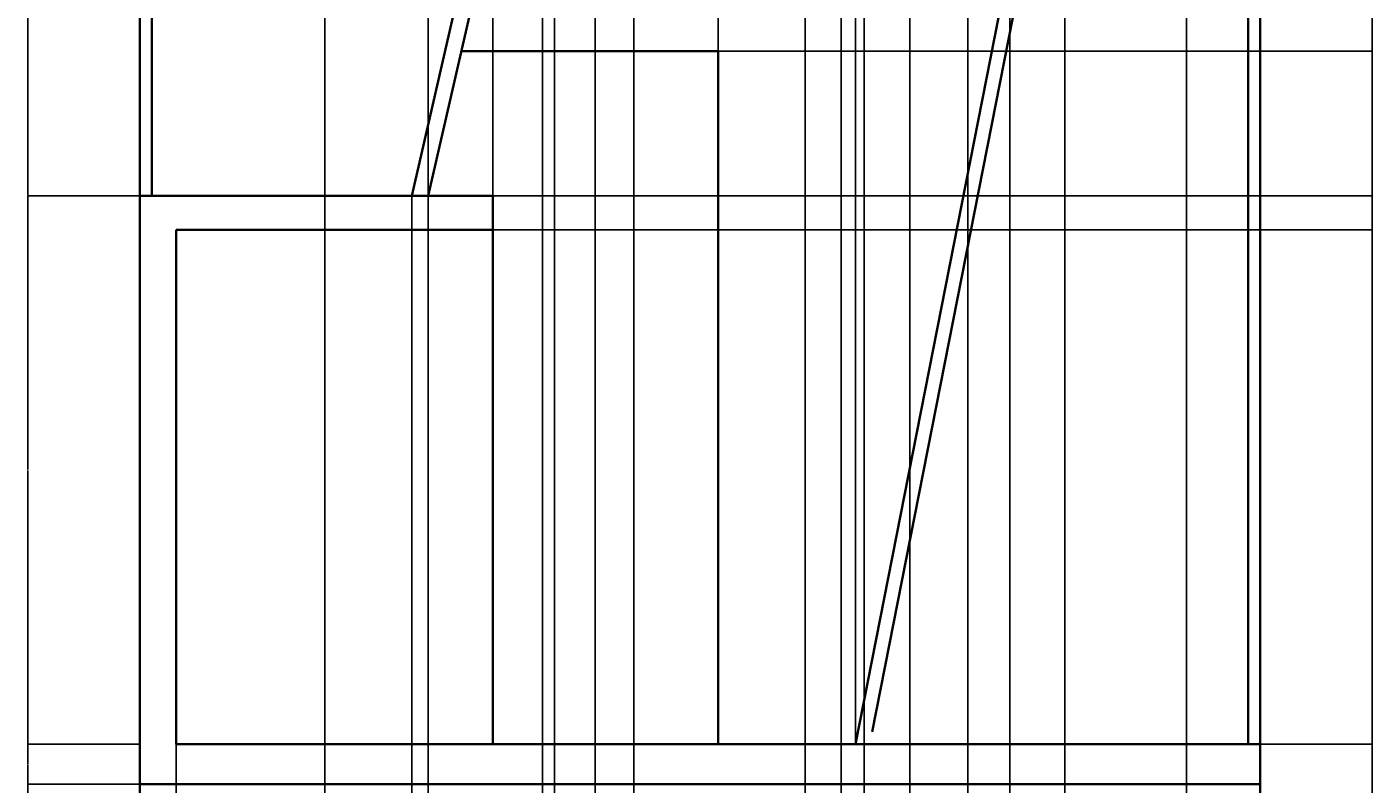
# Model space of a CAD drawing. Units: feet. Extents: x 2373 to 3800, y 799 to 1842.
# Tile 3 of 4: x 3224 to 3800, y 1129 to 1453. Entities that reach past the tile are written whole.
import ezdxf

# ---------------------------------------------------------------- set-up
doc = ezdxf.new("R2010")
doc.units = ezdxf.units.FT
doc.layers.add('A-ANNO-DIMS', color=2, linetype='Continuous', lineweight=18)
doc.layers.add('A-ELEV', color=7, linetype='Continuous', lineweight=35)
doc.styles.get("Standard").update_dxf_attribs({"font": 'arial.ttf'})
doc.dimstyles.get("Standard").update_dxf_attribs({"dimtxt": 0.18, "dimasz": 0.18, "dimexe": 0.18, "dimexo": 0.0625, "dimgap": 0.09, "dimtad": 0, "dimtih": 1, "dimtoh": 1, "dimdec": 1, "dimzin": 0, "dimdsep": 46, "dimlunit": 3, "dimtxsty": 'Standard', "dimcen": 0.09, "dimadec": 0, "dimazin": 0, "dimtfac": 1, "dimtdec": 1, "dimtofl": 0, "dimtmove": 0, "dimatfit": 3, "dimfxl": 1, "dimtolj": 1, "dimtzin": 0, "dimarcsym": 0})

# ---------------------------------------------------------------- blocks, each defined once
blk = doc.blocks.new('*D8')
at = {"layer": 'A-ANNO-DIMS', "color": 0, "lineweight": -2, "transparency": 16777216}
for p, q in [((3752.05, 1793.54), (3800.17, 1793.54)), ((3799.99, 1793.36), (3799.99, 1320.78)), ((3799.99, 847.83), (3799.99, 1320.41)), ((3752.05, 847.65), (3800.17, 847.65))]:
    blk.add_line(p, q, dxfattribs=at)
at = {"layer": 'A-ANNO-DIMS', "color": 0, "transparency": 16777216}
for points in [[(3799.96, 1793.36), (3800.02, 1793.36), (3799.99, 1793.54)], [(3799.96, 847.83), (3800.02, 847.83), (3799.99, 847.65)]]:
    blk.add_solid(points, dxfattribs=at)
at = {"layer": 'Defpoints', "color": 0, "transparency": 16777216}
for p in [(3751.99, 1793.54), (3799.99, 1793.54), (3751.99, 847.65)]:
    blk.add_point(p, dxfattribs=at)
at = {"layer": 'A-ANNO-DIMS', "color": 0, "transparency": 16777216, "insert": (3799.99, 1320.6), "char_height": 0.18, "attachment_point": 5}
blk.add_mtext('\\A1;945.9', dxfattribs=at)
blk = doc.blocks.new('*D9')
at = {"layer": 'A-ANNO-DIMS', "color": 0, "lineweight": -2, "transparency": 16777216}
for p, q in [((3271.92, 1128.67), (3223.81, 1128.67)), ((3223.99, 1128.49), (3223.99, 988.34)), ((3223.99, 847.83), (3223.99, 987.98)), ((3271.92, 847.65), (3223.81, 847.65))]:
    blk.add_line(p, q, dxfattribs=at)
at = {"layer": 'A-ANNO-DIMS', "color": 0, "transparency": 16777216}
for points in [[(3223.96, 1128.49), (3224.02, 1128.49), (3223.99, 1128.67)], [(3223.96, 847.83), (3224.02, 847.83), (3223.99, 847.65)]]:
    blk.add_solid(points, dxfattribs=at)
at = {"layer": 'Defpoints', "color": 0, "transparency": 16777216}
for p in [(3223.99, 1128.67), (3271.99, 1128.67), (3271.99, 847.65)]:
    blk.add_point(p, dxfattribs=at)
at = {"layer": 'A-ANNO-DIMS', "color": 0, "transparency": 16777216, "insert": (3223.99, 988.16), "char_height": 0.18, "attachment_point": 5}
blk.add_mtext('\\A1;281', dxfattribs=at)
blk = doc.blocks.new('*D10')
at = {"layer": 'A-ANNO-DIMS', "color": 0, "lineweight": -2, "transparency": 16777216}
for p, q in [((3271.92, 1145.79), (3223.81, 1145.79)), ((3223.99, 1145.61), (3223.99, 1137.41)), ((3223.99, 1128.85), (3223.99, 1137.05)), ((3271.92, 1128.67), (3223.81, 1128.67))]:
    blk.add_line(p, q, dxfattribs=at)
at = {"layer": 'A-ANNO-DIMS', "color": 0, "transparency": 16777216}
for points in [[(3223.96, 1145.61), (3224.02, 1145.61), (3223.99, 1145.79)], [(3223.96, 1128.85), (3224.02, 1128.85), (3223.99, 1128.67)]]:
    blk.add_solid(points, dxfattribs=at)
at = {"layer": 'Defpoints', "color": 0, "transparency": 16777216}
for p in [(3223.99, 1145.79), (3271.99, 1145.79), (3271.99, 1128.67)]:
    blk.add_point(p, dxfattribs=at)
at = {"layer": 'A-ANNO-DIMS', "color": 0, "transparency": 16777216, "insert": (3223.99, 1137.23), "char_height": 0.18, "attachment_point": 5}
blk.add_mtext('\\A1;17.12', dxfattribs=at)
blk = doc.blocks.new('*D11')
at = {"layer": 'A-ANNO-DIMS', "color": 0, "lineweight": -2, "transparency": 16777216}
for p, q in [((3271.92, 1380.85), (3223.81, 1380.85)), ((3223.99, 1380.67), (3223.99, 1263.5)), ((3223.99, 1145.97), (3223.99, 1263.14)), ((3271.92, 1145.79), (3223.81, 1145.79))]:
    blk.add_line(p, q, dxfattribs=at)
at = {"layer": 'A-ANNO-DIMS', "color": 0, "transparency": 16777216}
for points in [[(3223.96, 1380.67), (3224.02, 1380.67), (3223.99, 1380.85)], [(3223.96, 1145.97), (3224.02, 1145.97), (3223.99, 1145.79)]]:
    blk.add_solid(points, dxfattribs=at)
at = {"layer": 'Defpoints', "color": 0, "transparency": 16777216}
for p in [(3223.99, 1380.85), (3271.99, 1380.85), (3271.99, 1145.79)]:
    blk.add_point(p, dxfattribs=at)
at = {"layer": 'A-ANNO-DIMS', "color": 0, "transparency": 16777216, "insert": (3223.99, 1263.32), "char_height": 0.18, "attachment_point": 5}
blk.add_mtext('\\A1;235.06', dxfattribs=at)
blk = doc.blocks.new('*D12')
at = {"layer": 'A-ANNO-DIMS', "color": 0, "lineweight": -2, "transparency": 16777216}
for p, q in [((3271.92, 1672.17), (3223.81, 1672.17)), ((3223.99, 1671.99), (3223.99, 1526.69)), ((3223.99, 1381.03), (3223.99, 1526.33)), ((3271.92, 1380.85), (3223.81, 1380.85))]:
    blk.add_line(p, q, dxfattribs=at)
at = {"layer": 'A-ANNO-DIMS', "color": 0, "transparency": 16777216}
for points in [[(3223.96, 1671.99), (3224.02, 1671.99), (3223.99, 1672.17)], [(3223.96, 1381.03), (3224.02, 1381.03), (3223.99, 1380.85)]]:
    blk.add_solid(points, dxfattribs=at)
at = {"layer": 'Defpoints', "color": 0, "transparency": 16777216}
for p in [(3223.99, 1672.17), (3271.99, 1672.17), (3271.99, 1380.85)]:
    blk.add_point(p, dxfattribs=at)
at = {"layer": 'A-ANNO-DIMS', "color": 0, "transparency": 16777216, "insert": (3223.99, 1526.51), "char_height": 0.18, "attachment_point": 5}
blk.add_mtext('\\A1;291.3', dxfattribs=at)
blk = doc.blocks.new('*D13')
at = {"layer": 'A-ANNO-DIMS', "color": 0, "lineweight": -2, "transparency": 16777216}
for p, q in [((3271.99, 1380.91), (3271.99, 1841.72)), ((3272.17, 1841.54), (3347.21, 1841.54)), ((3423.01, 1841.54), (3347.97, 1841.54)), ((3423.19, 1380.91), (3423.19, 1841.72))]:
    blk.add_line(p, q, dxfattribs=at)
at = {"layer": 'A-ANNO-DIMS', "color": 0, "transparency": 16777216}
for points in [[(3272.17, 1841.57), (3272.17, 1841.51), (3271.99, 1841.54)], [(3423.01, 1841.57), (3423.01, 1841.51), (3423.19, 1841.54)]]:
    blk.add_solid(points, dxfattribs=at)
at = {"layer": 'Defpoints', "color": 0, "transparency": 16777216}
for p in [(3423.19, 1841.54), (3271.99, 1380.85), (3423.19, 1380.85)]:
    blk.add_point(p, dxfattribs=at)
at = {"layer": 'A-ANNO-DIMS', "color": 0, "transparency": 16777216, "insert": (3347.59, 1841.54), "char_height": 0.18, "attachment_point": 5}
blk.add_mtext('\\A1;151.2', dxfattribs=at)
blk = doc.blocks.new('*D14')
at = {"layer": 'A-ANNO-DIMS', "color": 0, "lineweight": -2, "transparency": 16777216}
for p, q in [((3423.19, 1145.85), (3423.19, 1841.72)), ((3423.37, 1841.54), (3471.07, 1841.54)), ((3519.56, 1841.54), (3471.86, 1841.54)), ((3519.74, 1442.83), (3519.74, 1841.72))]:
    blk.add_line(p, q, dxfattribs=at)
at = {"layer": 'A-ANNO-DIMS', "color": 0, "transparency": 16777216}
for points in [[(3423.37, 1841.57), (3423.37, 1841.51), (3423.19, 1841.54)], [(3519.56, 1841.57), (3519.56, 1841.51), (3519.74, 1841.54)]]:
    blk.add_solid(points, dxfattribs=at)
at = {"layer": 'Defpoints', "color": 0, "transparency": 16777216}
for p in [(3519.74, 1841.54), (3519.74, 1442.77), (3423.19, 1145.79)]:
    blk.add_point(p, dxfattribs=at)
at = {"layer": 'A-ANNO-DIMS', "color": 0, "transparency": 16777216, "insert": (3471.46, 1841.54), "char_height": 0.18, "attachment_point": 5}
blk.add_mtext('\\A1;96.54', dxfattribs=at)
blk = doc.blocks.new('*D15')
at = {"layer": 'A-ANNO-DIMS', "color": 0, "lineweight": -2, "transparency": 16777216}
for p, q in [((3519.8, 1442.77), (3800.17, 1442.77)), ((3799.99, 1442.59), (3799.99, 1294.46)), ((3799.99, 1145.97), (3799.99, 1294.1)), ((3519.8, 1145.79), (3800.17, 1145.79))]:
    blk.add_line(p, q, dxfattribs=at)
at = {"layer": 'A-ANNO-DIMS', "color": 0, "transparency": 16777216}
for points in [[(3799.96, 1442.59), (3800.02, 1442.59), (3799.99, 1442.77)], [(3799.96, 1145.97), (3800.02, 1145.97), (3799.99, 1145.79)]]:
    blk.add_solid(points, dxfattribs=at)
at = {"layer": 'Defpoints', "color": 0, "transparency": 16777216}
for p in [(3519.74, 1442.77), (3519.74, 1145.79), (3799.99, 1145.79)]:
    blk.add_point(p, dxfattribs=at)
at = {"layer": 'A-ANNO-DIMS', "color": 0, "transparency": 16777216, "insert": (3799.99, 1294.28), "char_height": 0.18, "attachment_point": 5}
blk.add_mtext('\\A1;297', dxfattribs=at)
blk = doc.blocks.new('*D17')
at = {"layer": 'A-ANNO-DIMS', "color": 0, "lineweight": -2, "transparency": 16777216}
for p, q in [((3666.72, 1562.42), (3800.17, 1562.42)), ((3799.99, 1562.24), (3799.99, 1354.28)), ((3799.99, 1145.97), (3799.99, 1353.92)), ((3578.6, 1145.79), (3800.17, 1145.79))]:
    blk.add_line(p, q, dxfattribs=at)
at = {"layer": 'A-ANNO-DIMS', "color": 0, "transparency": 16777216}
for points in [[(3799.96, 1562.24), (3800.02, 1562.24), (3799.99, 1562.42)], [(3799.96, 1145.97), (3800.02, 1145.97), (3799.99, 1145.79)]]:
    blk.add_solid(points, dxfattribs=at)
at = {"layer": 'Defpoints', "color": 0, "transparency": 16777216}
for p in [(3666.66, 1562.42), (3799.99, 1562.42), (3578.54, 1145.79)]:
    blk.add_point(p, dxfattribs=at)
at = {"layer": 'A-ANNO-DIMS', "color": 0, "transparency": 16777216, "insert": (3799.99, 1354.1), "char_height": 0.18, "attachment_point": 5}
blk.add_mtext('\\A1;416.6', dxfattribs=at)
blk = doc.blocks.new('*D20')
at = {"layer": 'A-ANNO-DIMS', "color": 0, "lineweight": -2, "transparency": 16777216}
for p, q in [((3572.43, 945.53), (3572.43, 1841.72)), ((3572.61, 1841.54), (3645.95, 1841.54)), ((3720.2, 1841.54), (3646.87, 1841.54)), ((3720.38, 1113.42), (3720.38, 1841.72))]:
    blk.add_line(p, q, dxfattribs=at)
at = {"layer": 'A-ANNO-DIMS', "color": 0, "transparency": 16777216}
for points in [[(3572.61, 1841.57), (3572.61, 1841.51), (3572.43, 1841.54)], [(3720.2, 1841.57), (3720.2, 1841.51), (3720.38, 1841.54)]]:
    blk.add_solid(points, dxfattribs=at)
at = {"layer": 'Defpoints', "color": 0, "transparency": 16777216}
for p in [(3720.38, 1841.54), (3720.38, 1113.36), (3572.43, 945.46)]:
    blk.add_point(p, dxfattribs=at)
at = {"layer": 'A-ANNO-DIMS', "color": 0, "transparency": 16777216, "insert": (3646.41, 1841.54), "char_height": 0.18, "attachment_point": 5}
blk.add_mtext('\\A1;147.95', dxfattribs=at)
blk = doc.blocks.new('*D23')
at = {"layer": 'A-ANNO-DIMS', "color": 0, "lineweight": -2, "transparency": 16777216}
for p, q in [((3483.65, 925.75), (3483.65, 1841.72)), ((3483.83, 1841.54), (3519.95, 1841.54)), ((3556.84, 1841.54), (3520.73, 1841.54)), ((3557.02, 1097.65), (3557.02, 1841.72))]:
    blk.add_line(p, q, dxfattribs=at)
at = {"layer": 'A-ANNO-DIMS', "color": 0, "transparency": 16777216}
for points in [[(3483.83, 1841.57), (3483.83, 1841.51), (3483.65, 1841.54)], [(3556.84, 1841.57), (3556.84, 1841.51), (3557.02, 1841.54)]]:
    blk.add_solid(points, dxfattribs=at)
at = {"layer": 'Defpoints', "color": 0, "transparency": 16777216}
for p in [(3557.02, 1841.54), (3557.02, 1097.59), (3483.65, 925.69)]:
    blk.add_point(p, dxfattribs=at)
at = {"layer": 'A-ANNO-DIMS', "color": 0, "transparency": 16777216, "insert": (3520.34, 1841.54), "char_height": 0.18, "attachment_point": 5}
blk.add_mtext('\\A1;73.37', dxfattribs=at)
blk = doc.blocks.new('*D27')
at = {"layer": 'A-ANNO-DIMS', "color": 0, "lineweight": -2, "transparency": 16777216}
for p, q in [((3444.52, 1624.82), (3444.52, 799.47)), ((3449.58, 1616.05), (3449.58, 799.47)), ((3444.7, 799.65), (3446.65, 799.65)), ((3449.4, 799.65), (3447.44, 799.65))]:
    blk.add_line(p, q, dxfattribs=at)
at = {"layer": 'A-ANNO-DIMS', "color": 0, "transparency": 16777216}
for points in [[(3444.7, 799.68), (3444.7, 799.62), (3444.52, 799.65)], [(3449.4, 799.68), (3449.4, 799.62), (3449.58, 799.65)]]:
    blk.add_solid(points, dxfattribs=at)
at = {"layer": 'Defpoints', "color": 0, "transparency": 16777216}
for p in [(3444.52, 1624.88), (3449.58, 1616.11), (3449.58, 799.65)]:
    blk.add_point(p, dxfattribs=at)
at = {"layer": 'A-ANNO-DIMS', "color": 0, "transparency": 16777216, "insert": (3447.05, 799.65), "char_height": 0.18, "attachment_point": 5}
blk.add_mtext('\\A1;5.057', dxfattribs=at)
blk = doc.blocks.new('*D28')
at = {"layer": 'A-ANNO-DIMS', "color": 0, "lineweight": -2, "transparency": 16777216}
for p, q in [((3271.99, 1380.79), (3271.99, 799.47)), ((3388.52, 1380.79), (3388.52, 799.47)), ((3272.17, 799.65), (3329.8, 799.65)), ((3388.34, 799.65), (3330.71, 799.65))]:
    blk.add_line(p, q, dxfattribs=at)
at = {"layer": 'A-ANNO-DIMS', "color": 0, "transparency": 16777216}
for points in [[(3272.17, 799.68), (3272.17, 799.62), (3271.99, 799.65)], [(3388.34, 799.68), (3388.34, 799.62), (3388.52, 799.65)]]:
    blk.add_solid(points, dxfattribs=at)
at = {"layer": 'Defpoints', "color": 0, "transparency": 16777216}
for p in [(3271.99, 1380.85), (3388.52, 1380.85), (3388.52, 799.65)]:
    blk.add_point(p, dxfattribs=at)
at = {"layer": 'A-ANNO-DIMS', "color": 0, "transparency": 16777216, "insert": (3330.25, 799.65), "char_height": 0.18, "attachment_point": 5}
blk.add_mtext('\\A1;116.53', dxfattribs=at)
blk = doc.blocks.new('*D29')
at = {"layer": 'A-ANNO-DIMS', "color": 0, "lineweight": -2, "transparency": 16777216}
for p, q in [((3519.74, 1145.85), (3519.74, 1841.72)), ((3519.92, 1841.54), (3548.81, 1841.54)), ((3578.36, 1841.54), (3549.46, 1841.54)), ((3578.54, 1145.85), (3578.54, 1841.72))]:
    blk.add_line(p, q, dxfattribs=at)
at = {"layer": 'A-ANNO-DIMS', "color": 0, "transparency": 16777216}
for points in [[(3519.92, 1841.57), (3519.92, 1841.51), (3519.74, 1841.54)], [(3578.36, 1841.57), (3578.36, 1841.51), (3578.54, 1841.54)]]:
    blk.add_solid(points, dxfattribs=at)
at = {"layer": 'Defpoints', "color": 0, "transparency": 16777216}
for p in [(3578.54, 1841.54), (3519.74, 1145.79), (3578.54, 1145.79)]:
    blk.add_point(p, dxfattribs=at)
at = {"layer": 'A-ANNO-DIMS', "color": 0, "transparency": 16777216, "insert": (3549.14, 1841.54), "char_height": 0.18, "attachment_point": 5}
blk.add_mtext('\\A1;58.8', dxfattribs=at)
blk = doc.blocks.new('*D30')
at = {"layer": 'A-ANNO-DIMS', "color": 0, "lineweight": -2, "transparency": 16777216}
for p, q in [((3271.99, 1366.11), (3271.99, 799.47)), ((3287.49, 1366.11), (3287.49, 799.47)), ((3272.17, 799.65), (3279.42, 799.65)), ((3287.31, 799.65), (3280.05, 799.65))]:
    blk.add_line(p, q, dxfattribs=at)
at = {"layer": 'A-ANNO-DIMS', "color": 0, "transparency": 16777216}
for points in [[(3272.17, 799.68), (3272.17, 799.62), (3271.99, 799.65)], [(3287.31, 799.68), (3287.31, 799.62), (3287.49, 799.65)]]:
    blk.add_solid(points, dxfattribs=at)
at = {"layer": 'Defpoints', "color": 0, "transparency": 16777216}
for p in [(3271.99, 1366.18), (3287.49, 1366.18), (3287.49, 799.65)]:
    blk.add_point(p, dxfattribs=at)
at = {"layer": 'A-ANNO-DIMS', "color": 0, "transparency": 16777216, "insert": (3279.74, 799.65), "char_height": 0.18, "attachment_point": 5}
blk.add_mtext('\\A1;15.5', dxfattribs=at)
blk = doc.blocks.new('*D31')
at = {"layer": 'A-ANNO-DIMS', "color": 0, "lineweight": -2, "transparency": 16777216}
for p, q in [((3277.19, 1380.85), (3800.17, 1380.85)), ((3799.99, 1380.67), (3799.99, 1373.69)), ((3799.99, 1366.36), (3799.99, 1373.33)), ((3287.55, 1366.18), (3800.17, 1366.18))]:
    blk.add_line(p, q, dxfattribs=at)
at = {"layer": 'A-ANNO-DIMS', "color": 0, "transparency": 16777216}
for points in [[(3799.96, 1380.67), (3800.02, 1380.67), (3799.99, 1380.85)], [(3799.96, 1366.36), (3800.02, 1366.36), (3799.99, 1366.18)]]:
    blk.add_solid(points, dxfattribs=at)
at = {"layer": 'Defpoints', "color": 0, "transparency": 16777216}
for p in [(3277.13, 1380.85), (3799.99, 1380.85), (3287.49, 1366.18)]:
    blk.add_point(p, dxfattribs=at)
at = {"layer": 'A-ANNO-DIMS', "color": 0, "transparency": 16777216, "insert": (3799.99, 1373.51), "char_height": 0.18, "attachment_point": 5}
blk.add_mtext('\\A1;14.674', dxfattribs=at)
blk = doc.blocks.new('*D36')
at = {"layer": 'A-ANNO-DIMS', "color": 0, "lineweight": -2, "transparency": 16777216}
for p, q in [((3351.18, 1010.48), (3351.18, 1841.72)), ((3351.36, 1841.54), (3372.95, 1841.54)), ((3395.3, 1841.54), (3373.71, 1841.54)), ((3395.48, 1010.48), (3395.48, 1841.72))]:
    blk.add_line(p, q, dxfattribs=at)
at = {"layer": 'A-ANNO-DIMS', "color": 0, "transparency": 16777216}
for points in [[(3351.36, 1841.57), (3351.36, 1841.51), (3351.18, 1841.54)], [(3395.3, 1841.57), (3395.3, 1841.51), (3395.48, 1841.54)]]:
    blk.add_solid(points, dxfattribs=at)
at = {"layer": 'Defpoints', "color": 0, "transparency": 16777216}
for p in [(3395.48, 1841.54), (3351.18, 1010.41), (3395.48, 1010.41)]:
    blk.add_point(p, dxfattribs=at)
at = {"layer": 'A-ANNO-DIMS', "color": 0, "transparency": 16777216, "insert": (3373.33, 1841.54), "char_height": 0.18, "attachment_point": 5}
blk.add_mtext('\\A1;44.31', dxfattribs=at)
blk = doc.blocks.new('*D37')
at = {"layer": 'A-ANNO-DIMS', "color": 0, "lineweight": -2, "transparency": 16777216}
for p, q in [((3395.48, 1097.65), (3395.48, 1841.72)), ((3395.66, 1841.54), (3430.91, 1841.54)), ((3466.94, 1841.54), (3431.69, 1841.54)), ((3467.12, 1097.65), (3467.12, 1841.72))]:
    blk.add_line(p, q, dxfattribs=at)
at = {"layer": 'A-ANNO-DIMS', "color": 0, "transparency": 16777216}
for points in [[(3395.66, 1841.57), (3395.66, 1841.51), (3395.48, 1841.54)], [(3466.94, 1841.57), (3466.94, 1841.51), (3467.12, 1841.54)]]:
    blk.add_solid(points, dxfattribs=at)
at = {"layer": 'Defpoints', "color": 0, "transparency": 16777216}
for p in [(3467.12, 1841.54), (3395.48, 1097.59), (3467.12, 1097.59)]:
    blk.add_point(p, dxfattribs=at)
at = {"layer": 'A-ANNO-DIMS', "color": 0, "transparency": 16777216, "insert": (3431.3, 1841.54), "char_height": 0.18, "attachment_point": 5}
blk.add_mtext('\\A1;71.63', dxfattribs=at)
blk = doc.blocks.new('*D38')
at = {"layer": 'A-ANNO-DIMS', "color": 0, "lineweight": -2, "transparency": 16777216}
for p, q in [((3467.12, 1097.65), (3467.12, 1841.72)), ((3467.3, 1841.54), (3474.93, 1841.54)), ((3483.47, 1841.54), (3475.84, 1841.54)), ((3483.65, 1097.65), (3483.65, 1841.72))]:
    blk.add_line(p, q, dxfattribs=at)
at = {"layer": 'A-ANNO-DIMS', "color": 0, "transparency": 16777216}
for points in [[(3467.3, 1841.57), (3467.3, 1841.51), (3467.12, 1841.54)], [(3483.47, 1841.57), (3483.47, 1841.51), (3483.65, 1841.54)]]:
    blk.add_solid(points, dxfattribs=at)
at = {"layer": 'Defpoints', "color": 0, "transparency": 16777216}
for p in [(3483.65, 1841.54), (3467.12, 1097.59), (3483.65, 1097.59)]:
    blk.add_point(p, dxfattribs=at)
at = {"layer": 'A-ANNO-DIMS', "color": 0, "transparency": 16777216, "insert": (3475.39, 1841.54), "char_height": 0.18, "attachment_point": 5}
blk.add_mtext('\\A1;16.537', dxfattribs=at)
blk = doc.blocks.new('*D48')
at = {"layer": 'A-ANNO-DIMS', "color": 0, "lineweight": -2, "transparency": 16777216}
for p, q in [((3582.33, 1693.47), (3582.33, 799.47)), ((3601.88, 1658.52), (3601.88, 799.47)), ((3582.51, 799.65), (3591.72, 799.65)), ((3601.7, 799.65), (3592.49, 799.65))]:
    blk.add_line(p, q, dxfattribs=at)
at = {"layer": 'A-ANNO-DIMS', "color": 0, "transparency": 16777216}
for points in [[(3582.51, 799.68), (3582.51, 799.62), (3582.33, 799.65)], [(3601.7, 799.68), (3601.7, 799.62), (3601.88, 799.65)]]:
    blk.add_solid(points, dxfattribs=at)
at = {"layer": 'Defpoints', "color": 0, "transparency": 16777216}
for p in [(3582.33, 1693.53), (3601.88, 1658.58), (3601.88, 799.65)]:
    blk.add_point(p, dxfattribs=at)
at = {"layer": 'A-ANNO-DIMS', "color": 0, "transparency": 16777216, "insert": (3592.11, 799.65), "char_height": 0.18, "attachment_point": 5}
blk.add_mtext('\\A1;19.55', dxfattribs=at)
blk = doc.blocks.new('*D49')
at = {"layer": 'A-ANNO-DIMS', "color": 0, "lineweight": -2, "transparency": 16777216}
for p, q in [((3626.67, 1690.12), (3626.67, 799.47)), ((3601.88, 1658.52), (3601.88, 799.47)), ((3602.06, 799.65), (3613.88, 799.65)), ((3626.49, 799.65), (3614.67, 799.65))]:
    blk.add_line(p, q, dxfattribs=at)
at = {"layer": 'A-ANNO-DIMS', "color": 0, "transparency": 16777216}
for points in [[(3602.06, 799.68), (3602.06, 799.62), (3601.88, 799.65)], [(3626.49, 799.68), (3626.49, 799.62), (3626.67, 799.65)]]:
    blk.add_solid(points, dxfattribs=at)
at = {"layer": 'Defpoints', "color": 0, "transparency": 16777216}
for p in [(3626.67, 1690.18), (3601.88, 1658.58), (3626.67, 799.65)]:
    blk.add_point(p, dxfattribs=at)
at = {"layer": 'A-ANNO-DIMS', "color": 0, "transparency": 16777216, "insert": (3614.28, 799.65), "char_height": 0.18, "attachment_point": 5}
blk.add_mtext('\\A1;24.79', dxfattribs=at)
blk = doc.blocks.new('*D50')
at = {"layer": 'A-ANNO-DIMS', "color": 0, "lineweight": -2, "transparency": 16777216}
for p, q in [((3626.67, 1690.12), (3626.67, 799.47)), ((3644.71, 1657.64), (3644.71, 799.47)), ((3626.85, 799.65), (3635.31, 799.65)), ((3644.53, 799.65), (3636.08, 799.65))]:
    blk.add_line(p, q, dxfattribs=at)
at = {"layer": 'A-ANNO-DIMS', "color": 0, "transparency": 16777216}
for points in [[(3626.85, 799.68), (3626.85, 799.62), (3626.67, 799.65)], [(3644.53, 799.68), (3644.53, 799.62), (3644.71, 799.65)]]:
    blk.add_solid(points, dxfattribs=at)
at = {"layer": 'Defpoints', "color": 0, "transparency": 16777216}
for p in [(3626.67, 1690.18), (3644.71, 1657.7), (3644.71, 799.65)]:
    blk.add_point(p, dxfattribs=at)
at = {"layer": 'A-ANNO-DIMS', "color": 0, "transparency": 16777216, "insert": (3635.69, 799.65), "char_height": 0.18, "attachment_point": 5}
blk.add_mtext('\\A1;18.03', dxfattribs=at)
blk = doc.blocks.new('*D51')
at = {"layer": 'A-ANNO-DIMS', "color": 0, "lineweight": -2, "transparency": 16777216}
for p, q in [((3644.71, 1657.64), (3644.71, 799.47)), ((3668.27, 1625.1), (3668.27, 799.47)), ((3644.89, 799.65), (3656.02, 799.65)), ((3668.09, 799.65), (3656.95, 799.65))]:
    blk.add_line(p, q, dxfattribs=at)
at = {"layer": 'A-ANNO-DIMS', "color": 0, "transparency": 16777216}
for points in [[(3644.89, 799.68), (3644.89, 799.62), (3644.71, 799.65)], [(3668.09, 799.68), (3668.09, 799.62), (3668.27, 799.65)]]:
    blk.add_solid(points, dxfattribs=at)
at = {"layer": 'Defpoints', "color": 0, "transparency": 16777216}
for p in [(3644.71, 1657.7), (3668.27, 1625.17), (3668.27, 799.65)]:
    blk.add_point(p, dxfattribs=at)
at = {"layer": 'A-ANNO-DIMS', "color": 0, "transparency": 16777216, "insert": (3656.49, 799.65), "char_height": 0.18, "attachment_point": 5}
blk.add_mtext('\\A1;23.567', dxfattribs=at)

msp = doc.modelspace()

# ---------------------------------------------------------------- linework, layer by layer
at = {"layer": 'A-ELEV'}
for p, q in [((3751.9863, 847.6543), (3751.9863, 1793.536)), ((3746.8473, 1785.9513), (3746.8473, 1145.7869)), ((3271.9863, 847.6543), (3271.9863, 1672.168)), ((3277.1253, 1667.1821), (3277.1253, 1380.85)), ((3444.5198, 1624.879), (3388.5169, 1380.85)), ((3449.5772, 1616.114), (3395.5857, 1380.85)), ((3585.7283, 1151.1084), (3666.6576, 1562.4189)), ((3578.5393, 1145.7869), (3659.4686, 1557.0974))]:
    msp.add_line(p, q, dxfattribs=at)
for points in [[(3409.7956, 1442.7685), (3519.7369, 1442.7685)], [(3519.7369, 1442.7685), (3519.7369, 1145.7869), (3423.1927, 1145.7869), (3423.1927, 1380.85)], [(3388.5169, 1380.85), (3271.9863, 1380.85), (3271.9863, 1128.6662), (3287.4874, 1128.6662)], [(3271.9863, 1366.1757), (3271.9863, 1380.85)], [(3388.5169, 1380.85), (3423.1927, 1380.85), (3423.1927, 1366.1757), (3287.4874, 1366.1757)], [(3287.4874, 1145.7869), (3287.4874, 1366.1757)], [(3271.9863, 1145.7869), (3271.9863, 1128.6662), (3751.9863, 1128.6662), (3751.9863, 1145.7869), (3287.4874, 1145.7869)]]:
    msp.add_lwpolyline(points, dxfattribs=at)

# ---------------------------------------------------------------- dimensions: what is measured, and where the dimension line sits
at = {"layer": 'A-ANNO-DIMS'}
for base, p1, p2, override, picture, middle in [((3423.1927, 1841.536), (3271.9863, 1380.85), (3423.1927, 1380.85), {"dimdec": 1, "dimlfac": 1, "dimrnd": 0, "dimzin": 0, "dimdsep": 46, "dimlunit": 2}, '*D13', (3347.5895, 1841.536)), ((3395.4819, 1841.536), (3351.1757, 1010.4128), (3395.4819, 1010.4128), {"dimdec": 2, "dimlfac": 1, "dimrnd": 0, "dimzin": 0, "dimdsep": 46, "dimlunit": 2}, '*D36', (3373.3288, 1841.536)), ((3467.1168, 1841.536), (3395.4819, 1097.5868), (3467.1168, 1097.5868), {"dimdec": 2, "dimlfac": 1, "dimrnd": 0, "dimzin": 0, "dimdsep": 46, "dimlunit": 2}, '*D37', (3431.2994, 1841.536)), ((3519.7369, 1841.536), (3423.1927, 1145.7869), (3519.7369, 1442.7685), {"dimdec": 2, "dimlfac": 1, "dimrnd": 0, "dimzin": 0, "dimdsep": 46, "dimlunit": 2}, '*D14', (3471.4648, 1841.536)), ((3483.65428, 1841.53598), (3467.11683, 1097.58685), (3483.65428, 1097.58685), {"dimdec": 3, "dimlfac": 1, "dimrnd": 0, "dimzin": 0, "dimdsep": 46, "dimlunit": 2}, '*D38', (3475.38556, 1841.53598)), ((3557.0236, 1841.536), (3483.6543, 925.687), (3557.0236, 1097.5868), {"dimdec": 2, "dimlfac": 1, "dimrnd": 0, "dimzin": 0, "dimdsep": 46, "dimlunit": 2}, '*D23', (3520.339, 1841.536)), ((3578.5393, 1841.536), (3519.7369, 1145.7869), (3578.5393, 1145.7869), {"dimdec": 1, "dimlfac": 1, "dimrnd": 0, "dimzin": 0, "dimdsep": 46, "dimlunit": 2}, '*D29', (3549.1381, 1841.536)), ((3720.385, 1841.536), (3572.4337, 945.465), (3720.385, 1113.3603), {"dimdec": 2, "dimlfac": 1, "dimrnd": 0, "dimzin": 0, "dimdsep": 46, "dimlunit": 2}, '*D20', (3646.4093, 1841.536)), ((3601.8833, 799.6543), (3582.3341, 1693.5326), (3601.8833, 1658.579), {"dimdec": 2, "dimlfac": 1, "dimrnd": 0, "dimzin": 0, "dimdsep": 46, "dimlunit": 2}, '*D48', (3592.1087, 799.6543)), ((3626.6744, 799.6543), (3601.8833, 1658.579), (3626.6744, 1690.1846), {"dimdec": 2, "dimlfac": 1, "dimrnd": 0, "dimzin": 0, "dimdsep": 46, "dimlunit": 2}, '*D49', (3614.2788, 799.6543)), ((3644.7062, 799.6543), (3626.6744, 1690.1846), (3644.7062, 1657.7009), {"dimdec": 2, "dimlfac": 1, "dimrnd": 0, "dimzin": 0, "dimdsep": 46, "dimlunit": 2}, '*D50', (3635.6903, 799.6543)), ((3668.2731, 799.6543), (3644.7062, 1657.7009), (3668.2731, 1625.1666), {"dimdec": 3, "dimlfac": 1, "dimrnd": 0, "dimzin": 0, "dimdsep": 46, "dimlunit": 2}, '*D51', (3656.4896, 799.6543)), ((3449.5772, 799.6543), (3444.5198, 1624.879), (3449.5772, 1616.114), {"dimdec": 3, "dimlfac": 1, "dimrnd": 0, "dimzin": 0, "dimdsep": 46, "dimlunit": 2}, '*D27', (3447.0485, 799.6543)), ((3388.5169, 799.6543), (3271.9863, 1380.85), (3388.5169, 1380.85), {"dimdec": 2, "dimlfac": 1, "dimrnd": 0, "dimzin": 0, "dimdsep": 46, "dimlunit": 2}, '*D28', (3330.2516, 799.6543)), ((3287.4874, 799.6543), (3271.9863, 1366.1757), (3287.4874, 1366.1757), {"dimdec": 1, "dimlfac": 1, "dimrnd": 0, "dimzin": 0, "dimdsep": 46, "dimlunit": 2}, '*D30', (3279.7369, 799.6543))]:
    dim = msp.add_linear_dim(base=base, p1=p1, p2=p2, dimstyle='Standard', override=override, dxfattribs=at)
    dim.commit()
    dim.dimension.update_dxf_attribs({"geometry": picture, "text_midpoint": middle})
for base, p1, p2, override, picture, middle in [((3799.9863, 1793.536), (3751.9863, 847.6543), (3751.9863, 1793.536), {"dimdec": 1, "dimlfac": 1, "dimrnd": 0, "dimzin": 0, "dimdsep": 46, "dimlunit": 2}, '*D8', (3799.9863, 1320.5951)), ((3223.9863, 1672.168), (3271.9863, 1380.85), (3271.9863, 1672.168), {"dimdec": 1, "dimlfac": 1, "dimrnd": 0, "dimzin": 0, "dimdsep": 46, "dimlunit": 2}, '*D12', (3223.9863, 1526.509)), ((3799.9863, 1562.4189), (3578.5393, 1145.7869), (3666.6576, 1562.4189), {"dimdec": 1, "dimlfac": 1, "dimrnd": 0, "dimzin": 0, "dimdsep": 46, "dimlunit": 2}, '*D17', (3799.9863, 1354.1029)), ((3799.9863, 1145.7869), (3519.7369, 1442.7685), (3519.7369, 1145.7869), {"dimdec": 0, "dimlfac": 1, "dimrnd": 0, "dimzin": 0, "dimdsep": 46, "dimlunit": 2}, '*D15', (3799.9863, 1294.2777)), ((3223.9863, 1380.85), (3271.9863, 1145.7869), (3271.9863, 1380.85), {"dimdec": 2, "dimlfac": 1, "dimrnd": 0, "dimzin": 0, "dimdsep": 46, "dimlunit": 2}, '*D11', (3223.9863, 1263.3184)), ((3799.9863, 1380.85), (3287.4874, 1366.1757), (3277.1253, 1380.85), {"dimdec": 3, "dimlfac": 1, "dimrnd": 0, "dimzin": 0, "dimdsep": 46, "dimlunit": 2}, '*D31', (3799.9863, 1373.5129)), ((3223.9863, 1145.7869), (3271.9863, 1128.6662), (3271.9863, 1145.7869), {"dimdec": 2, "dimlfac": 1, "dimrnd": 0, "dimzin": 0, "dimdsep": 46, "dimlunit": 2}, '*D10', (3223.9863, 1137.2265)), ((3223.9863, 1128.6662), (3271.9863, 847.6543), (3271.9863, 1128.6662), {"dimdec": 0, "dimlfac": 1, "dimrnd": 0, "dimzin": 0, "dimdsep": 46, "dimlunit": 2}, '*D9', (3223.9863, 988.1602))]:
    dim = msp.add_linear_dim(base=base, p1=p1, p2=p2, angle=90, dimstyle='Standard', override=override, dxfattribs=at)
    dim.commit()
    dim.dimension.update_dxf_attribs({"geometry": picture, "text_midpoint": middle})

doc.saveas('drawing.dxf')
